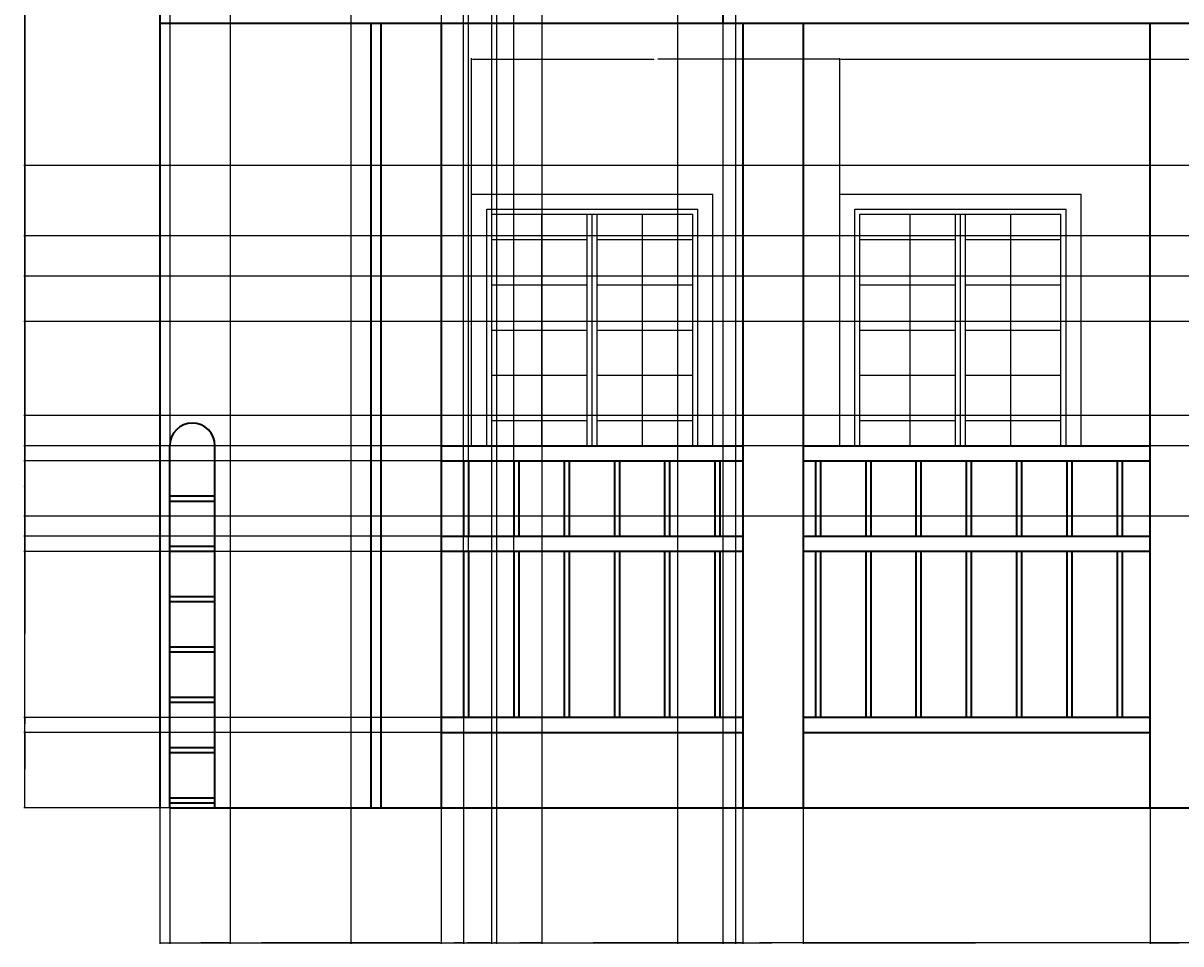
# Model space of a CAD drawing. Units: inches. Extents: x 2154 to 2740, y 571 to 1084.
# Tile 1 of 13: x 2154 to 2384, y 571 to 754. Entities that reach past the tile are written whole.
import ezdxf

# ---------------------------------------------------------------- set-up
doc = ezdxf.new("R2010")
doc.units = ezdxf.units.IN
for name, color, linetype, lineweight in [('A-ANNO-DIMS', 2, 'Continuous', 18), ('A-ELEV', 7, 'Continuous', 35), ('A-GLAZ', 4, 'Continuous', 25)]:
    doc.layers.add(name, color=color, linetype=linetype, lineweight=lineweight)
doc.styles.get("Standard").update_dxf_attribs({"font": 'arial.ttf'})
doc.dimstyles.get("Standard").update_dxf_attribs({"dimtxt": 0.18, "dimasz": 0.18, "dimexe": 0.18, "dimexo": 0.0625, "dimgap": 0.09, "dimtad": 0, "dimtih": 1, "dimtoh": 1, "dimdec": 4, "dimzin": 0, "dimdsep": 46, "dimtxsty": 'Standard', "dimcen": 0.09, "dimadec": 0, "dimazin": 0, "dimtfac": 1, "dimtdec": 4, "dimtofl": 0, "dimtmove": 0, "dimatfit": 3, "dimfxl": 1, "dimtolj": 1, "dimtzin": 0, "dimarcsym": 0})

# ---------------------------------------------------------------- blocks, each defined once
blk = doc.blocks.new('WIN-ELEV-1200')
for p, q in [((0, 50), (48, 50)), ((0, 0), (0, 50)), ((48, 0), (48, 50)), ((3, 0), (3, 47)), ((3, 47), (45, 47)), ((45, 0), (45, 47)), ((4, 46), (44, 46)), ((4, 0), (4, 46)), ((14, 0), (14, 46)), ((23, 0), (23, 46)), ((24, 0), (24, 46)), ((25, 0), (25, 46)), ((34, 0), (34, 46)), ((44, 0), (44, 46)), ((4, 41), (23, 41)), ((25, 41), (44, 41)), ((4, 32), (23, 32)), ((25, 32), (44, 32)), ((4, 23), (23, 23)), ((25, 23), (44, 23)), ((4, 14), (23, 14)), ((25, 14), (44, 14)), ((4, 5), (23, 5)), ((25, 5), (44, 5))]:
    blk.add_line(p, q)
blk = doc.blocks.new('*D10')
at = {"layer": 'A-ANNO-DIMS', "color": 0, "lineweight": -2, "transparency": 16777216}
for p, q in [((2447.14, 1057.01), (2154.18, 1057.01)), ((2154.36, 1056.83), (2154.36, 827.45)), ((2154.36, 597.71), (2154.36, 827.09)), ((2181.14, 597.53), (2154.18, 597.53))]:
    blk.add_line(p, q, dxfattribs=at)
at = {"layer": 'A-ANNO-DIMS', "color": 0, "transparency": 16777216}
for points in [[(2154.33, 1056.83), (2154.39, 1056.83), (2154.36, 1057.01)], [(2154.33, 597.71), (2154.39, 597.71), (2154.36, 597.53)]]:
    blk.add_solid(points, dxfattribs=at)
at = {"layer": 'Defpoints', "color": 0, "transparency": 16777216}
for p in [(2154.36, 1057.01), (2447.21, 1057.01), (2181.21, 597.53)]:
    blk.add_point(p, dxfattribs=at)
at = {"layer": 'A-ANNO-DIMS', "color": 0, "transparency": 16777216, "insert": (2154.36, 827.27), "char_height": 0.18, "attachment_point": 5}
blk.add_mtext('\\A1;459.5', dxfattribs=at)
blk = doc.blocks.new('*D14')
at = {"layer": 'A-ANNO-DIMS', "color": 0, "lineweight": -2, "transparency": 16777216}
for p, q in [((2221.14, 777.53), (2154.18, 777.53)), ((2154.36, 777.35), (2154.36, 687.71)), ((2154.36, 597.71), (2154.36, 687.35)), ((2223.14, 597.53), (2154.18, 597.53))]:
    blk.add_line(p, q, dxfattribs=at)
at = {"layer": 'A-ANNO-DIMS', "color": 0, "transparency": 16777216}
for points in [[(2154.33, 777.35), (2154.39, 777.35), (2154.36, 777.53)], [(2154.33, 597.71), (2154.39, 597.71), (2154.36, 597.53)]]:
    blk.add_solid(points, dxfattribs=at)
at = {"layer": 'Defpoints', "color": 0, "transparency": 16777216}
for p in [(2154.36, 777.53), (2221.21, 777.53), (2223.21, 597.53)]:
    blk.add_point(p, dxfattribs=at)
at = {"layer": 'A-ANNO-DIMS', "color": 0, "transparency": 16777216, "insert": (2154.36, 687.53), "char_height": 0.18, "attachment_point": 5}
blk.add_mtext('\\A1;180', dxfattribs=at)
blk = doc.blocks.new('*D16')
at = {"layer": 'A-ANNO-DIMS', "color": 0, "lineweight": -2, "transparency": 16777216}
for p, q in [((2181.21, 597.47), (2181.21, 570.5)), ((2237.21, 597.47), (2237.21, 570.5)), ((2181.39, 570.68), (2208.99, 570.68)), ((2237.03, 570.68), (2209.43, 570.68))]:
    blk.add_line(p, q, dxfattribs=at)
at = {"layer": 'A-ANNO-DIMS', "color": 0, "transparency": 16777216}
for points in [[(2181.39, 570.71), (2181.39, 570.65), (2181.21, 570.68)], [(2237.03, 570.71), (2237.03, 570.65), (2237.21, 570.68)]]:
    blk.add_solid(points, dxfattribs=at)
at = {"layer": 'Defpoints', "color": 0, "transparency": 16777216}
for p in [(2181.21, 597.53), (2237.21, 597.53), (2237.21, 570.68)]:
    blk.add_point(p, dxfattribs=at)
at = {"layer": 'A-ANNO-DIMS', "color": 0, "transparency": 16777216, "insert": (2209.21, 570.68), "char_height": 0.18, "attachment_point": 5}
blk.add_mtext('\\A1;56', dxfattribs=at)
blk = doc.blocks.new('*D17')
at = {"layer": 'A-ANNO-DIMS', "color": 0, "lineweight": -2, "transparency": 16777216}
for p, q in [((2237.21, 597.47), (2237.21, 570.5)), ((2297.21, 597.47), (2297.21, 570.5)), ((2237.39, 570.68), (2266.99, 570.68)), ((2297.03, 570.68), (2267.43, 570.68))]:
    blk.add_line(p, q, dxfattribs=at)
at = {"layer": 'A-ANNO-DIMS', "color": 0, "transparency": 16777216}
for points in [[(2237.39, 570.71), (2237.39, 570.65), (2237.21, 570.68)], [(2297.03, 570.71), (2297.03, 570.65), (2297.21, 570.68)]]:
    blk.add_solid(points, dxfattribs=at)
at = {"layer": 'Defpoints', "color": 0, "transparency": 16777216}
for p in [(2237.21, 597.53), (2297.21, 597.53), (2297.21, 570.68)]:
    blk.add_point(p, dxfattribs=at)
at = {"layer": 'A-ANNO-DIMS', "color": 0, "transparency": 16777216, "insert": (2267.21, 570.68), "char_height": 0.18, "attachment_point": 5}
blk.add_mtext('\\A1;60', dxfattribs=at)
blk = doc.blocks.new('*D18')
at = {"layer": 'A-ANNO-DIMS', "color": 0, "lineweight": -2, "transparency": 16777216}
for p, q in [((2297.21, 597.47), (2297.21, 570.5)), ((2309.21, 597.47), (2309.21, 570.5)), ((2297.39, 570.68), (2303, 570.68)), ((2309.03, 570.68), (2303.42, 570.68))]:
    blk.add_line(p, q, dxfattribs=at)
at = {"layer": 'A-ANNO-DIMS', "color": 0, "transparency": 16777216}
for points in [[(2297.39, 570.71), (2297.39, 570.65), (2297.21, 570.68)], [(2309.03, 570.71), (2309.03, 570.65), (2309.21, 570.68)]]:
    blk.add_solid(points, dxfattribs=at)
at = {"layer": 'Defpoints', "color": 0, "transparency": 16777216}
for p in [(2297.21, 597.53), (2309.21, 597.53), (2309.21, 570.68)]:
    blk.add_point(p, dxfattribs=at)
at = {"layer": 'A-ANNO-DIMS', "color": 0, "transparency": 16777216, "insert": (2303.21, 570.68), "char_height": 0.18, "attachment_point": 5}
blk.add_mtext('\\A1;12', dxfattribs=at)
blk = doc.blocks.new('*D19')
at = {"layer": 'A-ANNO-DIMS', "color": 0, "lineweight": -2, "transparency": 16777216}
for p, q in [((2309.21, 597.47), (2309.21, 570.5)), ((2378.21, 597.47), (2378.21, 570.5)), ((2309.39, 570.68), (2343.49, 570.68)), ((2378.03, 570.68), (2343.93, 570.68))]:
    blk.add_line(p, q, dxfattribs=at)
at = {"layer": 'A-ANNO-DIMS', "color": 0, "transparency": 16777216}
for points in [[(2309.39, 570.71), (2309.39, 570.65), (2309.21, 570.68)], [(2378.03, 570.71), (2378.03, 570.65), (2378.21, 570.68)]]:
    blk.add_solid(points, dxfattribs=at)
at = {"layer": 'Defpoints', "color": 0, "transparency": 16777216}
for p in [(2309.21, 597.53), (2378.21, 597.53), (2378.21, 570.68)]:
    blk.add_point(p, dxfattribs=at)
at = {"layer": 'A-ANNO-DIMS', "color": 0, "transparency": 16777216, "insert": (2343.71, 570.68), "char_height": 0.18, "attachment_point": 5}
blk.add_mtext('\\A1;69', dxfattribs=at)
blk = doc.blocks.new('*D20')
at = {"layer": 'A-ANNO-DIMS', "color": 0, "lineweight": -2, "transparency": 16777216}
for p, q in [((2378.21, 597.47), (2378.21, 570.5)), ((2390.21, 597.47), (2390.21, 570.5)), ((2378.39, 570.68), (2384, 570.68)), ((2390.03, 570.68), (2384.42, 570.68))]:
    blk.add_line(p, q, dxfattribs=at)
at = {"layer": 'A-ANNO-DIMS', "color": 0, "transparency": 16777216}
for points in [[(2378.39, 570.71), (2378.39, 570.65), (2378.21, 570.68)], [(2390.03, 570.71), (2390.03, 570.65), (2390.21, 570.68)]]:
    blk.add_solid(points, dxfattribs=at)
at = {"layer": 'Defpoints', "color": 0, "transparency": 16777216}
for p in [(2378.21, 597.53), (2390.21, 597.53), (2390.21, 570.68)]:
    blk.add_point(p, dxfattribs=at)
at = {"layer": 'A-ANNO-DIMS', "color": 0, "transparency": 16777216, "insert": (2384.21, 570.68), "char_height": 0.18, "attachment_point": 5}
blk.add_mtext('\\A1;12', dxfattribs=at)
blk = doc.blocks.new('*D29')
at = {"layer": 'A-ANNO-DIMS', "color": 0, "lineweight": -2, "transparency": 16777216}
for p, q in [((2657.14, 669.53), (2154.18, 669.53)), ((2154.36, 669.35), (2154.36, 633.71)), ((2154.36, 597.71), (2154.36, 633.35)), ((2657.14, 597.53), (2154.18, 597.53))]:
    blk.add_line(p, q, dxfattribs=at)
at = {"layer": 'A-ANNO-DIMS', "color": 0, "transparency": 16777216}
for points in [[(2154.33, 669.35), (2154.39, 669.35), (2154.36, 669.53)], [(2154.33, 597.71), (2154.39, 597.71), (2154.36, 597.53)]]:
    blk.add_solid(points, dxfattribs=at)
at = {"layer": 'Defpoints', "color": 0, "transparency": 16777216}
for p in [(2154.36, 669.53), (2657.21, 669.53), (2657.21, 597.53)]:
    blk.add_point(p, dxfattribs=at)
at = {"layer": 'A-ANNO-DIMS', "color": 0, "transparency": 16777216, "insert": (2154.36, 633.53), "char_height": 0.18, "attachment_point": 5}
blk.add_mtext('\\A1;72', dxfattribs=at)
blk = doc.blocks.new('*D31')
at = {"layer": 'A-ANNO-DIMS', "color": 0, "lineweight": -2, "transparency": 16777216}
for p, q in [((2421.64, 725.23), (2154.18, 725.23)), ((2154.36, 725.05), (2154.36, 661.56)), ((2154.36, 597.71), (2154.36, 661.2)), ((2417.14, 597.53), (2154.18, 597.53))]:
    blk.add_line(p, q, dxfattribs=at)
at = {"layer": 'A-ANNO-DIMS', "color": 0, "transparency": 16777216}
for points in [[(2154.33, 725.05), (2154.39, 725.05), (2154.36, 725.23)], [(2154.33, 597.71), (2154.39, 597.71), (2154.36, 597.53)]]:
    blk.add_solid(points, dxfattribs=at)
at = {"layer": 'Defpoints', "color": 0, "transparency": 16777216}
for p in [(2154.36, 725.23), (2421.71, 725.23), (2417.21, 597.53)]:
    blk.add_point(p, dxfattribs=at)
at = {"layer": 'A-ANNO-DIMS', "color": 0, "transparency": 16777216, "insert": (2154.36, 661.38), "char_height": 0.18, "attachment_point": 5}
blk.add_mtext('\\A1;127.7', dxfattribs=at)
blk = doc.blocks.new('*D39')
at = {"layer": 'A-ANNO-DIMS', "color": 0, "lineweight": -2, "transparency": 16777216}
for p, q in [((2183.21, 979.47), (2183.21, 570.5)), ((2417.21, 970.47), (2417.21, 570.5)), ((2183.39, 570.68), (2299.92, 570.68)), ((2417.03, 570.68), (2300.5, 570.68))]:
    blk.add_line(p, q, dxfattribs=at)
at = {"layer": 'A-ANNO-DIMS', "color": 0, "transparency": 16777216}
for points in [[(2183.39, 570.71), (2183.39, 570.65), (2183.21, 570.68)], [(2417.03, 570.71), (2417.03, 570.65), (2417.21, 570.68)]]:
    blk.add_solid(points, dxfattribs=at)
at = {"layer": 'Defpoints', "color": 0, "transparency": 16777216}
for p in [(2183.21, 979.53), (2417.21, 970.53), (2417.21, 570.68)]:
    blk.add_point(p, dxfattribs=at)
at = {"layer": 'A-ANNO-DIMS', "color": 0, "transparency": 16777216, "insert": (2300.21, 570.68), "char_height": 0.18, "attachment_point": 5}
blk.add_mtext('\\A1;234', dxfattribs=at)
blk = doc.blocks.new('*D43')
at = {"layer": 'A-ANNO-DIMS', "color": 0, "lineweight": -2, "transparency": 16777216}
for p, q in [((2243.26, 719.59), (2243.26, 746.56)), ((2243.44, 746.38), (2279.48, 746.38)), ((2316.32, 746.38), (2280.27, 746.38)), ((2316.5, 719.59), (2316.5, 746.56))]:
    blk.add_line(p, q, dxfattribs=at)
at = {"layer": 'A-ANNO-DIMS', "color": 0, "transparency": 16777216}
for points in [[(2243.44, 746.41), (2243.44, 746.35), (2243.26, 746.38)], [(2316.32, 746.41), (2316.32, 746.35), (2316.5, 746.38)]]:
    blk.add_solid(points, dxfattribs=at)
at = {"layer": 'Defpoints', "color": 0, "transparency": 16777216}
for p in [(2316.5, 746.38), (2243.26, 719.53), (2316.5, 719.53)]:
    blk.add_point(p, dxfattribs=at)
at = {"layer": 'A-ANNO-DIMS', "color": 0, "transparency": 16777216, "insert": (2279.88, 746.38), "char_height": 0.18, "attachment_point": 5}
blk.add_mtext('\\A1;73.24', dxfattribs=at)
blk = doc.blocks.new('*D44')
at = {"layer": 'A-ANNO-DIMS', "color": 0, "lineweight": -2, "transparency": 16777216}
for p, q in [((2316.5, 719.59), (2316.5, 746.56)), ((2316.68, 746.38), (2415.42, 746.38)), ((2515.07, 746.38), (2416.33, 746.38)), ((2515.25, 719.59), (2515.25, 746.56))]:
    blk.add_line(p, q, dxfattribs=at)
at = {"layer": 'A-ANNO-DIMS', "color": 0, "transparency": 16777216}
for points in [[(2316.68, 746.41), (2316.68, 746.35), (2316.5, 746.38)], [(2515.07, 746.41), (2515.07, 746.35), (2515.25, 746.38)]]:
    blk.add_solid(points, dxfattribs=at)
at = {"layer": 'Defpoints', "color": 0, "transparency": 16777216}
for p in [(2515.25, 746.38), (2316.5, 719.53), (2515.25, 719.53)]:
    blk.add_point(p, dxfattribs=at)
at = {"layer": 'A-ANNO-DIMS', "color": 0, "transparency": 16777216, "insert": (2415.87, 746.38), "char_height": 0.18, "attachment_point": 5}
blk.add_mtext('\\A1;198.75', dxfattribs=at)
blk = doc.blocks.new('*D51')
at = {"layer": 'A-ANNO-DIMS', "color": 0, "lineweight": -2, "transparency": 16777216}
for p, q in [((2183.21, 979.47), (2183.21, 570.5)), ((2195.21, 979.47), (2195.21, 570.5)), ((2183.39, 570.68), (2189, 570.68)), ((2195.03, 570.68), (2189.42, 570.68))]:
    blk.add_line(p, q, dxfattribs=at)
at = {"layer": 'A-ANNO-DIMS', "color": 0, "transparency": 16777216}
for points in [[(2183.39, 570.71), (2183.39, 570.65), (2183.21, 570.68)], [(2195.03, 570.71), (2195.03, 570.65), (2195.21, 570.68)]]:
    blk.add_solid(points, dxfattribs=at)
at = {"layer": 'Defpoints', "color": 0, "transparency": 16777216}
for p in [(2183.21, 979.53), (2195.21, 979.53), (2195.21, 570.68)]:
    blk.add_point(p, dxfattribs=at)
at = {"layer": 'A-ANNO-DIMS', "color": 0, "transparency": 16777216, "insert": (2189.21, 570.68), "char_height": 0.18, "attachment_point": 5}
blk.add_mtext('\\A1;12', dxfattribs=at)
blk = doc.blocks.new('*D52')
at = {"layer": 'A-ANNO-DIMS', "color": 0, "lineweight": -2, "transparency": 16777216}
for p, q in [((2284.21, 903.47), (2284.21, 570.5)), ((2293.21, 903.47), (2293.21, 570.5)), ((2284.39, 570.68), (2288.56, 570.68)), ((2293.03, 570.68), (2288.86, 570.68))]:
    blk.add_line(p, q, dxfattribs=at)
at = {"layer": 'A-ANNO-DIMS', "color": 0, "transparency": 16777216}
for points in [[(2284.39, 570.71), (2284.39, 570.65), (2284.21, 570.68)], [(2293.03, 570.71), (2293.03, 570.65), (2293.21, 570.68)]]:
    blk.add_solid(points, dxfattribs=at)
at = {"layer": 'Defpoints', "color": 0, "transparency": 16777216}
for p in [(2284.21, 903.53), (2293.21, 903.53), (2293.21, 570.68)]:
    blk.add_point(p, dxfattribs=at)
at = {"layer": 'A-ANNO-DIMS', "color": 0, "transparency": 16777216, "insert": (2288.71, 570.68), "char_height": 0.18, "attachment_point": 5}
blk.add_mtext('\\A1;9', dxfattribs=at)
blk = doc.blocks.new('*D56')
at = {"layer": 'A-ANNO-DIMS', "color": 0, "lineweight": -2, "transparency": 16777216}
for p, q in [((2293.21, 915.47), (2293.21, 570.5)), ((2295.77, 915.97), (2295.77, 570.5)), ((2293.39, 570.68), (2294.16, 570.68)), ((2295.59, 570.68), (2294.81, 570.68))]:
    blk.add_line(p, q, dxfattribs=at)
at = {"layer": 'A-ANNO-DIMS', "color": 0, "transparency": 16777216}
for points in [[(2293.39, 570.71), (2293.39, 570.65), (2293.21, 570.68)], [(2295.59, 570.71), (2295.59, 570.65), (2295.77, 570.68)]]:
    blk.add_solid(points, dxfattribs=at)
at = {"layer": 'Defpoints', "color": 0, "transparency": 16777216}
for p in [(2293.21, 915.53), (2295.77, 916.03), (2295.77, 570.68)]:
    blk.add_point(p, dxfattribs=at)
at = {"layer": 'A-ANNO-DIMS', "color": 0, "transparency": 16777216, "insert": (2294.49, 570.68), "char_height": 0.18, "attachment_point": 5}
blk.add_mtext('\\A1;2.56', dxfattribs=at)
blk = doc.blocks.new('*D61')
at = {"layer": 'A-ANNO-DIMS', "color": 0, "lineweight": -2, "transparency": 16777216}
for p, q in [((2183.21, 757.47), (2183.21, 570.5)), ((2219.21, 757.47), (2219.21, 570.5)), ((2183.39, 570.68), (2200.99, 570.68)), ((2219.03, 570.68), (2201.43, 570.68))]:
    blk.add_line(p, q, dxfattribs=at)
at = {"layer": 'A-ANNO-DIMS', "color": 0, "transparency": 16777216}
for points in [[(2183.39, 570.71), (2183.39, 570.65), (2183.21, 570.68)], [(2219.03, 570.71), (2219.03, 570.65), (2219.21, 570.68)]]:
    blk.add_solid(points, dxfattribs=at)
at = {"layer": 'Defpoints', "color": 0, "transparency": 16777216}
for p in [(2183.21, 757.53), (2219.21, 757.53), (2219.21, 570.68)]:
    blk.add_point(p, dxfattribs=at)
at = {"layer": 'A-ANNO-DIMS', "color": 0, "transparency": 16777216, "insert": (2201.21, 570.68), "char_height": 0.18, "attachment_point": 5}
blk.add_mtext('\\A1;36', dxfattribs=at)
blk = doc.blocks.new('*D95')
at = {"layer": 'A-ANNO-DIMS', "color": 0, "lineweight": -2, "transparency": 16777216}
for p, q in [((2435.64, 711.23), (2154.18, 711.23)), ((2154.36, 711.05), (2154.36, 707.41)), ((2154.36, 703.41), (2154.36, 707.05)), ((2439.64, 703.23), (2154.18, 703.23))]:
    blk.add_line(p, q, dxfattribs=at)
at = {"layer": 'A-ANNO-DIMS', "color": 0, "transparency": 16777216}
for points in [[(2154.33, 711.05), (2154.39, 711.05), (2154.36, 711.23)], [(2154.33, 703.41), (2154.39, 703.41), (2154.36, 703.23)]]:
    blk.add_solid(points, dxfattribs=at)
at = {"layer": 'Defpoints', "color": 0, "transparency": 16777216}
for p in [(2435.71, 711.23), (2154.36, 703.23), (2439.71, 703.23)]:
    blk.add_point(p, dxfattribs=at)
at = {"layer": 'A-ANNO-DIMS', "color": 0, "transparency": 16777216, "insert": (2154.36, 707.23), "char_height": 0.18, "attachment_point": 5}
blk.add_mtext('\\A1;8', dxfattribs=at)
blk = doc.blocks.new('*D96')
at = {"layer": 'A-ANNO-DIMS', "color": 0, "lineweight": -2, "transparency": 16777216}
for p, q in [((2439.64, 703.23), (2154.18, 703.23)), ((2154.36, 703.05), (2154.36, 698.91)), ((2154.36, 694.41), (2154.36, 698.55)), ((2435.64, 694.23), (2154.18, 694.23))]:
    blk.add_line(p, q, dxfattribs=at)
at = {"layer": 'A-ANNO-DIMS', "color": 0, "transparency": 16777216}
for points in [[(2154.33, 703.05), (2154.39, 703.05), (2154.36, 703.23)], [(2154.33, 694.41), (2154.39, 694.41), (2154.36, 694.23)]]:
    blk.add_solid(points, dxfattribs=at)
at = {"layer": 'Defpoints', "color": 0, "transparency": 16777216}
for p in [(2439.71, 703.23), (2154.36, 694.23), (2435.71, 694.23)]:
    blk.add_point(p, dxfattribs=at)
at = {"layer": 'A-ANNO-DIMS', "color": 0, "transparency": 16777216, "insert": (2154.36, 698.73), "char_height": 0.18, "attachment_point": 5}
blk.add_mtext('\\A1;9', dxfattribs=at)
blk = doc.blocks.new('*D98')
at = {"layer": 'A-ANNO-DIMS', "color": 0, "lineweight": -2, "transparency": 16777216}
for p, q in [((2408.14, 675.53), (2154.18, 675.53)), ((2154.36, 675.35), (2154.36, 665.71)), ((2154.36, 655.71), (2154.36, 665.35)), ((2408.14, 655.53), (2154.18, 655.53))]:
    blk.add_line(p, q, dxfattribs=at)
at = {"layer": 'A-ANNO-DIMS', "color": 0, "transparency": 16777216}
for points in [[(2154.33, 675.35), (2154.39, 675.35), (2154.36, 675.53)], [(2154.33, 655.71), (2154.39, 655.71), (2154.36, 655.53)]]:
    blk.add_solid(points, dxfattribs=at)
at = {"layer": 'Defpoints', "color": 0, "transparency": 16777216}
for p in [(2154.36, 675.53), (2408.21, 675.53), (2408.21, 655.53)]:
    blk.add_point(p, dxfattribs=at)
at = {"layer": 'A-ANNO-DIMS', "color": 0, "transparency": 16777216, "insert": (2154.36, 665.53), "char_height": 0.18, "attachment_point": 5}
blk.add_mtext('\\A1;20', dxfattribs=at)
blk = doc.blocks.new('*D126')
at = {"layer": 'A-ANNO-DIMS', "color": 0, "lineweight": -2, "transparency": 16777216}
for p, q in [((2237.21, 787.47), (2237.21, 570.5)), ((2247.21, 787.47), (2247.21, 570.5)), ((2237.39, 570.68), (2242, 570.68)), ((2247.03, 570.68), (2242.42, 570.68))]:
    blk.add_line(p, q, dxfattribs=at)
at = {"layer": 'A-ANNO-DIMS', "color": 0, "transparency": 16777216}
for points in [[(2237.39, 570.71), (2237.39, 570.65), (2237.21, 570.68)], [(2247.03, 570.71), (2247.03, 570.65), (2247.21, 570.68)]]:
    blk.add_solid(points, dxfattribs=at)
at = {"layer": 'Defpoints', "color": 0, "transparency": 16777216}
for p in [(2237.21, 787.53), (2247.21, 787.53), (2247.21, 570.68)]:
    blk.add_point(p, dxfattribs=at)
at = {"layer": 'A-ANNO-DIMS', "color": 0, "transparency": 16777216, "insert": (2242.21, 570.68), "char_height": 0.18, "attachment_point": 5}
blk.add_mtext('\\A1;10', dxfattribs=at)
blk = doc.blocks.new('*D127')
at = {"layer": 'A-ANNO-DIMS', "color": 0, "lineweight": -2, "transparency": 16777216}
for p, q in [((2247.21, 787.47), (2247.21, 570.5)), ((2248.21, 787.47), (2248.21, 570.5)), ((2247.39, 570.68), (2247.58, 570.68)), ((2248.03, 570.68), (2247.83, 570.68))]:
    blk.add_line(p, q, dxfattribs=at)
at = {"layer": 'A-ANNO-DIMS', "color": 0, "transparency": 16777216}
for points in [[(2247.39, 570.71), (2247.39, 570.65), (2247.21, 570.68)], [(2248.03, 570.71), (2248.03, 570.65), (2248.21, 570.68)]]:
    blk.add_solid(points, dxfattribs=at)
at = {"layer": 'Defpoints', "color": 0, "transparency": 16777216}
for p in [(2247.21, 787.53), (2248.21, 787.53), (2248.21, 570.68)]:
    blk.add_point(p, dxfattribs=at)
at = {"layer": 'A-ANNO-DIMS', "color": 0, "transparency": 16777216, "insert": (2247.71, 570.68), "char_height": 0.18, "attachment_point": 5}
blk.add_mtext('\\A1;1', dxfattribs=at)
blk = doc.blocks.new('*D128')
at = {"layer": 'A-ANNO-DIMS', "color": 0, "lineweight": -2, "transparency": 16777216}
for p, q in [((2248.21, 787.47), (2248.21, 570.5)), ((2257.21, 787.47), (2257.21, 570.5)), ((2248.39, 570.68), (2252.56, 570.68)), ((2257.03, 570.68), (2252.86, 570.68))]:
    blk.add_line(p, q, dxfattribs=at)
at = {"layer": 'A-ANNO-DIMS', "color": 0, "transparency": 16777216}
for points in [[(2248.39, 570.71), (2248.39, 570.65), (2248.21, 570.68)], [(2257.03, 570.71), (2257.03, 570.65), (2257.21, 570.68)]]:
    blk.add_solid(points, dxfattribs=at)
at = {"layer": 'Defpoints', "color": 0, "transparency": 16777216}
for p in [(2248.21, 787.53), (2257.21, 787.53), (2257.21, 570.68)]:
    blk.add_point(p, dxfattribs=at)
at = {"layer": 'A-ANNO-DIMS', "color": 0, "transparency": 16777216, "insert": (2252.71, 570.68), "char_height": 0.18, "attachment_point": 5}
blk.add_mtext('\\A1;9', dxfattribs=at)
blk = doc.blocks.new('*D129')
at = {"layer": 'A-ANNO-DIMS', "color": 0, "lineweight": -2, "transparency": 16777216}
for p, q in [((2237.14, 612.53), (2154.18, 612.53)), ((2154.36, 612.35), (2154.36, 605.21)), ((2154.36, 597.71), (2154.36, 604.85)), ((2237.14, 597.53), (2154.18, 597.53))]:
    blk.add_line(p, q, dxfattribs=at)
at = {"layer": 'A-ANNO-DIMS', "color": 0, "transparency": 16777216}
for points in [[(2154.33, 612.35), (2154.39, 612.35), (2154.36, 612.53)], [(2154.33, 597.71), (2154.39, 597.71), (2154.36, 597.53)]]:
    blk.add_solid(points, dxfattribs=at)
at = {"layer": 'Defpoints', "color": 0, "transparency": 16777216}
for p in [(2154.36, 612.53), (2237.21, 612.53), (2237.21, 597.53)]:
    blk.add_point(p, dxfattribs=at)
at = {"layer": 'A-ANNO-DIMS', "color": 0, "transparency": 16777216, "insert": (2154.36, 605.03), "char_height": 0.18, "attachment_point": 5}
blk.add_mtext('\\A1;15', dxfattribs=at)
blk = doc.blocks.new('*D130')
at = {"layer": 'A-ANNO-DIMS', "color": 0, "lineweight": -2, "transparency": 16777216}
for p, q in [((2237.14, 615.53), (2154.18, 615.53)), ((2154.36, 615.35), (2154.36, 614.21)), ((2154.36, 612.71), (2154.36, 613.85)), ((2237.14, 612.53), (2154.18, 612.53))]:
    blk.add_line(p, q, dxfattribs=at)
at = {"layer": 'A-ANNO-DIMS', "color": 0, "transparency": 16777216}
for points in [[(2154.33, 615.35), (2154.39, 615.35), (2154.36, 615.53)], [(2154.33, 612.71), (2154.39, 612.71), (2154.36, 612.53)]]:
    blk.add_solid(points, dxfattribs=at)
at = {"layer": 'Defpoints', "color": 0, "transparency": 16777216}
for p in [(2154.36, 615.53), (2237.21, 615.53), (2237.21, 612.53)]:
    blk.add_point(p, dxfattribs=at)
at = {"layer": 'A-ANNO-DIMS', "color": 0, "transparency": 16777216, "insert": (2154.36, 614.03), "char_height": 0.18, "attachment_point": 5}
blk.add_mtext('\\A1;3', dxfattribs=at)
blk = doc.blocks.new('*D131')
at = {"layer": 'A-ANNO-DIMS', "color": 0, "lineweight": -2, "transparency": 16777216}
for p, q in [((2237.14, 648.53), (2154.18, 648.53)), ((2154.36, 648.35), (2154.36, 632.21)), ((2154.36, 615.71), (2154.36, 631.85)), ((2237.14, 615.53), (2154.18, 615.53))]:
    blk.add_line(p, q, dxfattribs=at)
at = {"layer": 'A-ANNO-DIMS', "color": 0, "transparency": 16777216}
for points in [[(2154.33, 648.35), (2154.39, 648.35), (2154.36, 648.53)], [(2154.33, 615.71), (2154.39, 615.71), (2154.36, 615.53)]]:
    blk.add_solid(points, dxfattribs=at)
at = {"layer": 'Defpoints', "color": 0, "transparency": 16777216}
for p in [(2154.36, 648.53), (2237.21, 648.53), (2237.21, 615.53)]:
    blk.add_point(p, dxfattribs=at)
at = {"layer": 'A-ANNO-DIMS', "color": 0, "transparency": 16777216, "insert": (2154.36, 632.03), "char_height": 0.18, "attachment_point": 5}
blk.add_mtext('\\A1;33', dxfattribs=at)
blk = doc.blocks.new('*D132')
at = {"layer": 'A-ANNO-DIMS', "color": 0, "lineweight": -2, "transparency": 16777216}
for p, q in [((2237.14, 651.53), (2154.18, 651.53)), ((2154.36, 651.35), (2154.36, 650.21)), ((2154.36, 648.71), (2154.36, 649.85)), ((2237.14, 648.53), (2154.18, 648.53))]:
    blk.add_line(p, q, dxfattribs=at)
at = {"layer": 'A-ANNO-DIMS', "color": 0, "transparency": 16777216}
for points in [[(2154.33, 651.35), (2154.39, 651.35), (2154.36, 651.53)], [(2154.33, 648.71), (2154.39, 648.71), (2154.36, 648.53)]]:
    blk.add_solid(points, dxfattribs=at)
at = {"layer": 'Defpoints', "color": 0, "transparency": 16777216}
for p in [(2154.36, 651.53), (2237.21, 651.53), (2237.21, 648.53)]:
    blk.add_point(p, dxfattribs=at)
at = {"layer": 'A-ANNO-DIMS', "color": 0, "transparency": 16777216, "insert": (2154.36, 650.03), "char_height": 0.18, "attachment_point": 5}
blk.add_mtext('\\A1;3', dxfattribs=at)
blk = doc.blocks.new('*D133')
at = {"layer": 'A-ANNO-DIMS', "color": 0, "lineweight": -2, "transparency": 16777216}
for p, q in [((2237.14, 666.53), (2154.18, 666.53)), ((2154.36, 666.35), (2154.36, 659.21)), ((2154.36, 651.71), (2154.36, 658.85)), ((2237.14, 651.53), (2154.18, 651.53))]:
    blk.add_line(p, q, dxfattribs=at)
at = {"layer": 'A-ANNO-DIMS', "color": 0, "transparency": 16777216}
for points in [[(2154.33, 666.35), (2154.39, 666.35), (2154.36, 666.53)], [(2154.33, 651.71), (2154.39, 651.71), (2154.36, 651.53)]]:
    blk.add_solid(points, dxfattribs=at)
at = {"layer": 'Defpoints', "color": 0, "transparency": 16777216}
for p in [(2154.36, 666.53), (2237.21, 666.53), (2237.21, 651.53)]:
    blk.add_point(p, dxfattribs=at)
at = {"layer": 'A-ANNO-DIMS', "color": 0, "transparency": 16777216, "insert": (2154.36, 659.03), "char_height": 0.18, "attachment_point": 5}
blk.add_mtext('\\A1;15', dxfattribs=at)
blk = doc.blocks.new('*D134')
at = {"layer": 'A-ANNO-DIMS', "color": 0, "lineweight": -2, "transparency": 16777216}
for p, q in [((2237.14, 669.53), (2154.18, 669.53)), ((2154.36, 669.35), (2154.36, 668.21)), ((2154.36, 666.71), (2154.36, 667.85)), ((2237.14, 666.53), (2154.18, 666.53))]:
    blk.add_line(p, q, dxfattribs=at)
at = {"layer": 'A-ANNO-DIMS', "color": 0, "transparency": 16777216}
for points in [[(2154.33, 669.35), (2154.39, 669.35), (2154.36, 669.53)], [(2154.33, 666.71), (2154.39, 666.71), (2154.36, 666.53)]]:
    blk.add_solid(points, dxfattribs=at)
at = {"layer": 'Defpoints', "color": 0, "transparency": 16777216}
for p in [(2154.36, 669.53), (2237.21, 669.53), (2237.21, 666.53)]:
    blk.add_point(p, dxfattribs=at)
at = {"layer": 'A-ANNO-DIMS', "color": 0, "transparency": 16777216, "insert": (2154.36, 668.03), "char_height": 0.18, "attachment_point": 5}
blk.add_mtext('\\A1;3', dxfattribs=at)
blk = doc.blocks.new('*D135')
at = {"layer": 'A-ANNO-DIMS', "color": 0, "lineweight": -2, "transparency": 16777216}
for p, q in [((2241.65, 615.47), (2241.65, 570.5)), ((2237.21, 612.47), (2237.21, 570.5)), ((2237.39, 570.68), (2239.03, 570.68)), ((2241.47, 570.68), (2239.83, 570.68))]:
    blk.add_line(p, q, dxfattribs=at)
at = {"layer": 'A-ANNO-DIMS', "color": 0, "transparency": 16777216}
for points in [[(2237.39, 570.71), (2237.39, 570.65), (2237.21, 570.68)], [(2241.47, 570.71), (2241.47, 570.65), (2241.65, 570.68)]]:
    blk.add_solid(points, dxfattribs=at)
at = {"layer": 'Defpoints', "color": 0, "transparency": 16777216}
for p in [(2241.65, 615.53), (2237.21, 612.53), (2241.65, 570.68)]:
    blk.add_point(p, dxfattribs=at)
at = {"layer": 'A-ANNO-DIMS', "color": 0, "transparency": 16777216, "insert": (2239.43, 570.68), "char_height": 0.18, "attachment_point": 5}
blk.add_mtext('\\A1;4.446', dxfattribs=at)
blk = doc.blocks.new('*D136')
at = {"layer": 'A-ANNO-DIMS', "color": 0, "lineweight": -2, "transparency": 16777216}
for p, q in [((2241.65, 648.59), (2241.65, 1084.04)), ((2241.83, 1083.86), (2242.03, 1083.86)), ((2242.47, 1083.86), (2242.28, 1083.86)), ((2242.65, 648.59), (2242.65, 1084.04))]:
    blk.add_line(p, q, dxfattribs=at)
at = {"layer": 'A-ANNO-DIMS', "color": 0, "transparency": 16777216}
for points in [[(2241.83, 1083.89), (2241.83, 1083.83), (2241.65, 1083.86)], [(2242.47, 1083.89), (2242.47, 1083.83), (2242.65, 1083.86)]]:
    blk.add_solid(points, dxfattribs=at)
at = {"layer": 'Defpoints', "color": 0, "transparency": 16777216}
for p in [(2242.65, 1083.86), (2241.65, 648.53), (2242.65, 648.53)]:
    blk.add_point(p, dxfattribs=at)
at = {"layer": 'A-ANNO-DIMS', "color": 0, "transparency": 16777216, "insert": (2242.15, 1083.86), "char_height": 0.18, "attachment_point": 5}
blk.add_mtext('\\A1;1', dxfattribs=at)
blk = doc.blocks.new('*D137')
at = {"layer": 'A-ANNO-DIMS', "color": 0, "lineweight": -2, "transparency": 16777216}
for p, q in [((2242.65, 648.59), (2242.65, 1084.04)), ((2242.83, 1083.86), (2247, 1083.86)), ((2251.47, 1083.86), (2247.3, 1083.86)), ((2251.65, 648.59), (2251.65, 1084.04))]:
    blk.add_line(p, q, dxfattribs=at)
at = {"layer": 'A-ANNO-DIMS', "color": 0, "transparency": 16777216}
for points in [[(2242.83, 1083.89), (2242.83, 1083.83), (2242.65, 1083.86)], [(2251.47, 1083.89), (2251.47, 1083.83), (2251.65, 1083.86)]]:
    blk.add_solid(points, dxfattribs=at)
at = {"layer": 'Defpoints', "color": 0, "transparency": 16777216}
for p in [(2251.65, 1083.86), (2242.65, 648.53), (2251.65, 648.53)]:
    blk.add_point(p, dxfattribs=at)
at = {"layer": 'A-ANNO-DIMS', "color": 0, "transparency": 16777216, "insert": (2247.15, 1083.86), "char_height": 0.18, "attachment_point": 5}
blk.add_mtext('\\A1;9', dxfattribs=at)

msp = doc.modelspace()

# ---------------------------------------------------------------- linework, layer by layer
at = {"layer": 'A-ELEV'}
for p, q in [((2181.2067, 981.5321), (2181.2067, 753.5321)), ((2293.2067, 777.5321), (2293.2067, 753.5321)), ((2181.2067, 753.5321), (2713.2067, 753.5321)), ((2181.2067, 753.5321), (2181.2067, 597.5321)), ((2223.2067, 753.5321), (2223.2067, 597.5321)), ((2225.2067, 753.5321), (2225.2067, 597.5321)), ((2237.2067, 753.5321), (2237.2067, 597.5321)), ((2297.2067, 753.5321), (2297.2067, 597.5321)), ((2309.2067, 753.5321), (2309.2067, 597.5321)), ((2378.2067, 753.5321), (2378.2067, 597.5321)), ((2183.2067, 597.5321), (2183.2067, 669.5321)), ((2192.2067, 597.5321), (2192.2067, 669.5321)), ((2237.2067, 669.5321), (2297.2067, 669.5321)), ((2309.2067, 669.5321), (2378.2067, 669.5321)), ((2237.2067, 666.5321), (2297.2067, 666.5321)), ((2241.6527, 666.5321), (2241.6527, 651.5321)), ((2242.6527, 666.5321), (2242.6527, 651.5321)), ((2251.6527, 666.5321), (2251.6527, 651.5321)), ((2252.6527, 666.5321), (2252.6527, 651.5321)), ((2261.6527, 666.5321), (2261.6527, 651.5321)), ((2262.6527, 666.5321), (2262.6527, 651.5321)), ((2271.6527, 666.5321), (2271.6527, 651.5321)), ((2272.6527, 666.5321), (2272.6527, 651.5321)), ((2281.6527, 666.5321), (2281.6527, 651.5321)), ((2282.6527, 666.5321), (2282.6527, 651.5321)), ((2291.6527, 666.5321), (2291.6527, 651.5321)), ((2292.6527, 666.5321), (2292.6527, 651.5321)), ((2309.2067, 666.5321), (2378.2067, 666.5321)), ((2311.6527, 666.5321), (2311.6527, 651.5321)), ((2312.6527, 666.5321), (2312.6527, 651.5321)), ((2321.6527, 666.5321), (2321.6527, 651.5321)), ((2322.6527, 666.5321), (2322.6527, 651.5321)), ((2331.6527, 666.5321), (2331.6527, 651.5321)), ((2332.6527, 666.5321), (2332.6527, 651.5321)), ((2341.6527, 666.5321), (2341.6527, 651.5321)), ((2342.6527, 666.5321), (2342.6527, 651.5321)), ((2351.6527, 666.5321), (2351.6527, 651.5321)), ((2352.6527, 666.5321), (2352.6527, 651.5321)), ((2361.6527, 666.5321), (2361.6527, 651.5321)), ((2362.6527, 666.5321), (2362.6527, 651.5321)), ((2371.6527, 666.5321), (2371.6527, 651.5321)), ((2372.6527, 666.5321), (2372.6527, 651.5321)), ((2183.2067, 659.5321), (2192.2067, 659.5321)), ((2183.2067, 658.5321), (2192.2067, 658.5321)), ((2183.2067, 649.5321), (2192.2067, 649.5321)), ((2237.2067, 651.5321), (2297.2067, 651.5321)), ((2309.2067, 651.5321), (2378.2067, 651.5321)), ((2183.2067, 648.5321), (2192.2067, 648.5321)), ((2237.2067, 648.5321), (2297.2067, 648.5321)), ((2241.6527, 648.5321), (2241.6527, 615.5321)), ((2242.6527, 648.5321), (2242.6527, 615.5321)), ((2251.6527, 648.5321), (2251.6527, 615.5321)), ((2252.6527, 648.5321), (2252.6527, 615.5321)), ((2261.6527, 648.5321), (2261.6527, 615.5321)), ((2262.6527, 648.5321), (2262.6527, 615.5321)), ((2271.6527, 648.5321), (2271.6527, 615.5321)), ((2272.6527, 648.5321), (2272.6527, 615.5321)), ((2281.6527, 648.5321), (2281.6527, 615.5321)), ((2282.6527, 648.5321), (2282.6527, 615.5321)), ((2291.6527, 648.5321), (2291.6527, 615.5321)), ((2292.6527, 648.5321), (2292.6527, 615.5321)), ((2309.2067, 648.5321), (2378.2067, 648.5321)), ((2311.6527, 648.5321), (2311.6527, 615.5321)), ((2312.6527, 648.5321), (2312.6527, 615.5321)), ((2321.6527, 648.5321), (2321.6527, 615.5321)), ((2322.6527, 648.5321), (2322.6527, 615.5321)), ((2331.6527, 648.5321), (2331.6527, 615.5321)), ((2332.6527, 648.5321), (2332.6527, 615.5321)), ((2341.6527, 648.5321), (2341.6527, 615.5321)), ((2342.6527, 648.5321), (2342.6527, 615.5321)), ((2351.6527, 648.5321), (2351.6527, 615.5321)), ((2352.6527, 648.5321), (2352.6527, 615.5321)), ((2361.6527, 648.5321), (2361.6527, 615.5321)), ((2362.6527, 648.5321), (2362.6527, 615.5321)), ((2371.6527, 648.5321), (2371.6527, 615.5321)), ((2372.6527, 648.5321), (2372.6527, 615.5321)), ((2183.2067, 639.5321), (2192.2067, 639.5321)), ((2183.2067, 638.5321), (2192.2067, 638.5321)), ((2183.2067, 629.5321), (2192.2067, 629.5321)), ((2183.2067, 628.5321), (2192.2067, 628.5321)), ((2183.2067, 619.5321), (2192.2067, 619.5321)), ((2183.2067, 618.5321), (2192.2067, 618.5321)), ((2237.2067, 615.5321), (2297.2067, 615.5321)), ((2309.2067, 615.5321), (2378.2067, 615.5321)), ((2237.2067, 612.5321), (2297.2067, 612.5321)), ((2309.2067, 612.5321), (2378.2067, 612.5321)), ((2183.2067, 609.5321), (2192.2067, 609.5321)), ((2183.2067, 608.5321), (2192.2067, 608.5321)), ((2183.2067, 599.5321), (2192.2067, 599.5321)), ((2183.2067, 598.5321), (2192.2067, 598.5321)), ((2183.2067, 597.5321), (2713.2067, 597.5321)), ((2223.2067, 597.5321), (2671.2067, 597.5321))]:
    msp.add_line(p, q, dxfattribs=at)
msp.add_arc((2187.7067, 669.5321), 4.5, 0, 180, dxfattribs=at)

# ---------------------------------------------------------------- block references
at = {"layer": 'A-GLAZ'}
for p in [(2243.2571, 669.532), (2316.4978, 669.532)]:
    msp.add_blockref('WIN-ELEV-1200', p, dxfattribs=at)

# ---------------------------------------------------------------- dimensions: what is measured, and where the dimension line sits
at = {"layer": 'A-ANNO-DIMS'}
for base, p1, p2, override, picture, middle in [((2242.6527, 1083.8553), (2241.6527, 648.5321), (2242.6527, 648.5321), {"dimdec": 0, "dimlfac": 1, "dimrnd": 0, "dimzin": 0, "dimdsep": 46, "dimlunit": 2}, '*D136', (2242.1527, 1083.8553)), ((2251.6527, 1083.8553), (2242.6527, 648.5321), (2251.6527, 648.5321), {"dimdec": 0, "dimlfac": 1, "dimrnd": 0, "dimzin": 0, "dimdsep": 46, "dimlunit": 2}, '*D137', (2247.1527, 1083.8553)), ((2417.2067, 570.6821), (2183.2067, 979.5321), (2417.2067, 970.5321), {"dimdec": 0, "dimlfac": 1, "dimrnd": 0, "dimzin": 0, "dimdsep": 46, "dimlunit": 2}, '*D39', (2300.2067, 570.6821)), ((2195.2067, 570.6821), (2183.2067, 979.5321), (2195.2067, 979.5321), {"dimdec": 0, "dimlfac": 1, "dimrnd": 0, "dimzin": 0, "dimdsep": 46, "dimlunit": 2}, '*D51', (2189.2067, 570.6821)), ((2295.7714, 570.6821), (2293.2067, 915.5321), (2295.7714, 916.028), {"dimdec": 2, "dimlfac": 1, "dimrnd": 0, "dimzin": 0, "dimdsep": 46, "dimlunit": 2}, '*D56', (2294.4891, 570.6821)), ((2293.2067, 570.6821), (2284.2067, 903.5321), (2293.2067, 903.5321), {"dimdec": 0, "dimlfac": 1, "dimrnd": 0, "dimzin": 0, "dimdsep": 46, "dimlunit": 2}, '*D52', (2288.7067, 570.6821)), ((2247.2067, 570.6821), (2237.2067, 787.5321), (2247.2067, 787.5321), {"dimdec": 0, "dimlfac": 1, "dimrnd": 0, "dimzin": 0, "dimdsep": 46, "dimlunit": 2}, '*D126', (2242.2067, 570.6821)), ((2248.2067, 570.6821), (2247.2067, 787.5321), (2248.2067, 787.5321), {"dimdec": 0, "dimlfac": 1, "dimrnd": 0, "dimzin": 0, "dimdsep": 46, "dimlunit": 2}, '*D127', (2247.7067, 570.6821)), ((2257.2067, 570.6821), (2248.2067, 787.5321), (2257.2067, 787.5321), {"dimdec": 0, "dimlfac": 1, "dimrnd": 0, "dimzin": 0, "dimdsep": 46, "dimlunit": 2}, '*D128', (2252.7067, 570.6821)), ((2219.2067, 570.6821), (2183.2067, 757.5321), (2219.2067, 757.5321), {"dimdec": 0, "dimlfac": 1, "dimrnd": 0, "dimzin": 0, "dimdsep": 46, "dimlunit": 2}, '*D61', (2201.2067, 570.6821)), ((2316.4975, 746.3821), (2243.2568, 719.5321), (2316.4975, 719.5321), {"dimdec": 2, "dimlfac": 1, "dimrnd": 0, "dimzin": 0, "dimdsep": 46, "dimlunit": 2}, '*D43', (2279.8771, 746.3821)), ((2515.2489, 746.3821), (2316.4975, 719.5321), (2515.2489, 719.5321), {"dimdec": 2, "dimlfac": 1, "dimrnd": 0, "dimzin": 0, "dimdsep": 46, "dimlunit": 2}, '*D44', (2415.8732, 746.3821)), ((2241.6527, 570.6821), (2237.2067, 612.5321), (2241.6527, 615.5321), {"dimdec": 3, "dimlfac": 1, "dimrnd": 0, "dimzin": 0, "dimdsep": 46, "dimlunit": 2}, '*D135', (2239.4297, 570.6821)), ((2237.2067, 570.6821), (2181.2067, 597.5321), (2237.2067, 597.5321), {"dimdec": 0, "dimlfac": 1, "dimrnd": 0, "dimzin": 0, "dimdsep": 46, "dimlunit": 2}, '*D16', (2209.2067, 570.6821)), ((2297.2067, 570.6821), (2237.2067, 597.5321), (2297.2067, 597.5321), {"dimdec": 0, "dimlfac": 1, "dimrnd": 0, "dimzin": 0, "dimdsep": 46, "dimlunit": 2}, '*D17', (2267.2067, 570.6821)), ((2309.2067, 570.6821), (2297.2067, 597.5321), (2309.2067, 597.5321), {"dimdec": 0, "dimlfac": 1, "dimrnd": 0, "dimzin": 0, "dimdsep": 46, "dimlunit": 2}, '*D18', (2303.2067, 570.6821)), ((2378.2067, 570.6821), (2309.2067, 597.5321), (2378.2067, 597.5321), {"dimdec": 0, "dimlfac": 1, "dimrnd": 0, "dimzin": 0, "dimdsep": 46, "dimlunit": 2}, '*D19', (2343.7067, 570.6821)), ((2390.2067, 570.6821), (2378.2067, 597.5321), (2390.2067, 597.5321), {"dimdec": 0, "dimlfac": 1, "dimrnd": 0, "dimzin": 0, "dimdsep": 46, "dimlunit": 2}, '*D20', (2384.2067, 570.6821))]:
    dim = msp.add_linear_dim(base=base, p1=p1, p2=p2, dimstyle='Standard', override=override, dxfattribs=at)
    dim.commit()
    dim.dimension.update_dxf_attribs({"geometry": picture, "text_midpoint": middle})
for base, p1, p2, override, picture, middle in [((2154.3567, 1057.0053), (2181.2067, 597.5321), (2447.2067, 1057.0053), {"dimdec": 1, "dimlfac": 1, "dimrnd": 0, "dimzin": 0, "dimdsep": 46, "dimlunit": 2}, '*D10', (2154.3567, 827.2687)), ((2154.3567, 777.5321), (2223.2067, 597.5321), (2221.2067, 777.5321), {"dimdec": 0, "dimlfac": 1, "dimrnd": 0, "dimzin": 0, "dimdsep": 46, "dimlunit": 2}, '*D14', (2154.3567, 687.5321)), ((2154.3567, 725.2281), (2417.2067, 597.5321), (2421.7067, 725.2281), {"dimdec": 1, "dimlfac": 1, "dimrnd": 0, "dimzin": 0, "dimdsep": 46, "dimlunit": 2}, '*D31', (2154.3567, 661.3801)), ((2154.3567, 703.2281), (2435.7067, 711.2281), (2439.7067, 703.2281), {"dimdec": 0, "dimlfac": 1, "dimrnd": 0, "dimzin": 0, "dimdsep": 46, "dimlunit": 2}, '*D95', (2154.3567, 707.2281)), ((2154.3567, 694.2281), (2439.7067, 703.2281), (2435.7067, 694.2281), {"dimdec": 0, "dimlfac": 1, "dimrnd": 0, "dimzin": 0, "dimdsep": 46, "dimlunit": 2}, '*D96', (2154.3567, 698.7281)), ((2154.3567, 675.5321), (2408.2067, 655.5321), (2408.2067, 675.5321), {"dimdec": 0, "dimlfac": 1, "dimrnd": 0, "dimzin": 0, "dimdsep": 46, "dimlunit": 2}, '*D98', (2154.3567, 665.5321)), ((2154.3567, 669.5321), (2657.2067, 597.5321), (2657.2067, 669.5321), {"dimdec": 0, "dimlfac": 1, "dimrnd": 0, "dimzin": 0, "dimdsep": 46, "dimlunit": 2}, '*D29', (2154.3567, 633.5321)), ((2154.3567, 669.5321), (2237.2067, 666.5321), (2237.2067, 669.5321), {"dimdec": 0, "dimlfac": 1, "dimrnd": 0, "dimzin": 0, "dimdsep": 46, "dimlunit": 2}, '*D134', (2154.3567, 668.0321)), ((2154.3567, 666.5321), (2237.2067, 651.5321), (2237.2067, 666.5321), {"dimdec": 0, "dimlfac": 1, "dimrnd": 0, "dimzin": 0, "dimdsep": 46, "dimlunit": 2}, '*D133', (2154.3567, 659.0321)), ((2154.3567, 651.5321), (2237.2067, 648.5321), (2237.2067, 651.5321), {"dimdec": 0, "dimlfac": 1, "dimrnd": 0, "dimzin": 0, "dimdsep": 46, "dimlunit": 2}, '*D132', (2154.3567, 650.0321)), ((2154.3567, 648.5321), (2237.2067, 615.5321), (2237.2067, 648.5321), {"dimdec": 0, "dimlfac": 1, "dimrnd": 0, "dimzin": 0, "dimdsep": 46, "dimlunit": 2}, '*D131', (2154.3567, 632.0321)), ((2154.3567, 615.5321), (2237.2067, 612.5321), (2237.2067, 615.5321), {"dimdec": 0, "dimlfac": 1, "dimrnd": 0, "dimzin": 0, "dimdsep": 46, "dimlunit": 2}, '*D130', (2154.3567, 614.0321)), ((2154.3567, 612.5321), (2237.2067, 597.5321), (2237.2067, 612.5321), {"dimdec": 0, "dimlfac": 1, "dimrnd": 0, "dimzin": 0, "dimdsep": 46, "dimlunit": 2}, '*D129', (2154.3567, 605.0321))]:
    dim = msp.add_linear_dim(base=base, p1=p1, p2=p2, angle=90, dimstyle='Standard', override=override, dxfattribs=at)
    dim.commit()
    dim.dimension.update_dxf_attribs({"geometry": picture, "text_midpoint": middle})

doc.saveas('drawing.dxf')
